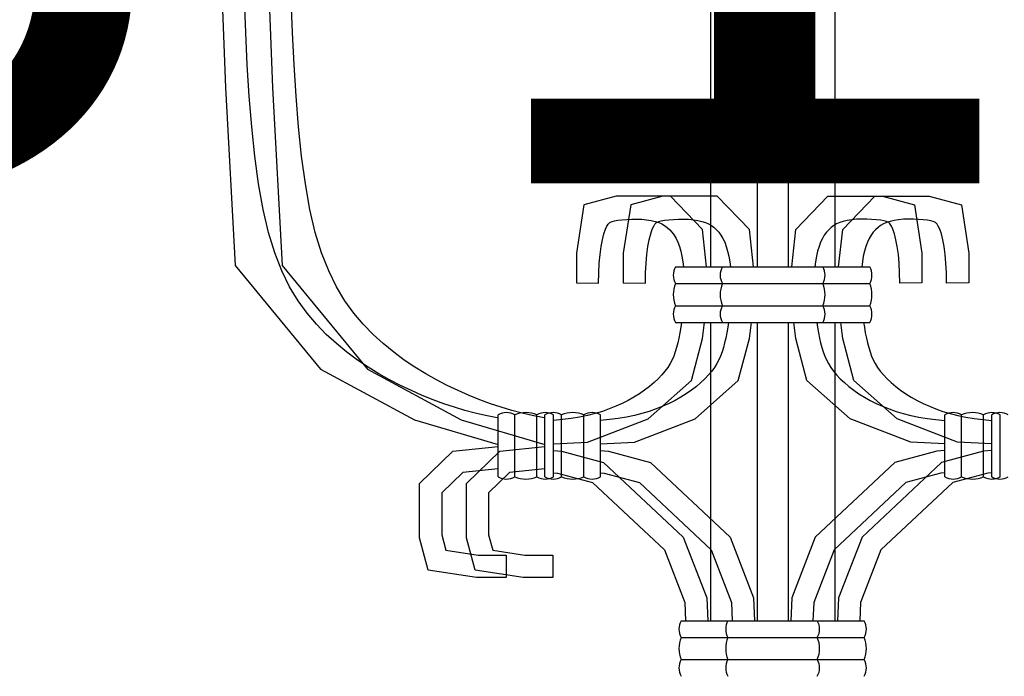
# Model space of a CAD drawing. Units: inches. Extents: x 2278 to 7495, y -71 to 1198.
# Tile 31 of 44: x 5127.04 to 5134.27, y 136.372 to 141.192. Entities that reach past the tile are written whole.
import ezdxf

# ---------------------------------------------------------------- set-up
doc = ezdxf.new("R2010")
doc.units = ezdxf.units.IN
doc.header["$MEASUREMENT"] = 0
doc.layers.add('A-ANNO-DIMS', color=2, linetype='Continuous', lineweight=18)
doc.layers.add('A-ELEV', color=7, linetype='Continuous', lineweight=25)
doc.styles.get("Standard").update_dxf_attribs({"font": 'arial.ttf'})
doc.dimstyles.get("Standard").update_dxf_attribs({"dimtxt": 6, "dimasz": 3, "dimexe": 0.18, "dimexo": 0.0625, "dimgap": 0.09, "dimtad": 0, "dimtih": 1, "dimtoh": 1, "dimdec": 0, "dimzin": 0, "dimdsep": 46, "dimlunit": 3, "dimtxsty": 'Standard', "dimblk": 'ARCHTICK', "dimcen": 0.09, "dimadec": 0, "dimazin": 0, "dimtfac": 1, "dimtdec": 0, "dimtofl": 0, "dimtmove": 0, "dimatfit": 3, "dimfxl": 1, "dimtolj": 1, "dimtzin": 0, "dimarcsym": 0})

# ---------------------------------------------------------------- blocks, each defined once
blk = doc.blocks.new('_ArchTick')
at = {"color": 0, "linetype": 'ByBlock', "const_width": 0.15}
blk.add_lwpolyline([(-0.5, -0.5), (0.5, 0.5)], dxfattribs=at)
blk = doc.blocks.new('*D59')
at = {"layer": 'A-ANNO-DIMS', "color": 0, "lineweight": -2, "transparency": 16777216}
for p, q in [((5096.5894, 159.1826), (5101.5644, 159.1826)), ((5101.3844, 159.1826), (5101.3844, 146.185)), ((5101.3844, 126.7988), (5101.3844, 139.7963)), ((5096.5894, 126.7988), (5101.5644, 126.7988))]:
    blk.add_line(p, q, dxfattribs=at)
at = {"layer": 'Defpoints', "color": 0, "transparency": 16777216}
for p in [(5096.5269, 159.1826), (5101.3844, 159.1826), (5096.5269, 126.7988)]:
    blk.add_point(p, dxfattribs=at)
at = {"layer": 'A-ANNO-DIMS', "color": 0, "lineweight": -2, "transparency": 16777216, "xscale": 3, "yscale": 3, "zscale": 3}
for p, rotation in [((5101.3844, 159.1826), 90), ((5101.3844, 126.7988), 270)]:
    blk.add_blockref('_ArchTick', p, dxfattribs=dict(at, rotation=rotation))
at = {"layer": 'A-ANNO-DIMS', "color": 0, "transparency": 16777216, "insert": (5101.3844, 142.9907), "char_height": 6, "attachment_point": 5}
blk.add_mtext('\\A1;ORNATE BALUSTER 2\'-8 1/2" TYP.', dxfattribs=at)
blk = doc.blocks.new('*D123')
at = {"layer": 'A-ANNO-DIMS', "color": 0, "lineweight": -2, "transparency": 16777216}
for p, q in [((4736.95, 340.1567), (4736.95, -23.4272)), ((5145.6762, -1.8097), (5145.6762, -23.4272)), ((4736.95, -23.2472), (4923.9291, -23.2472)), ((5145.6762, -23.2472), (4958.6971, -23.2472))]:
    blk.add_line(p, q, dxfattribs=at)
at = {"layer": 'Defpoints', "color": 0, "transparency": 16777216}
for p in [(4736.95, 340.2192), (5145.6762, -1.7472), (5145.6762, -23.2472)]:
    blk.add_point(p, dxfattribs=at)
at = {"layer": 'A-ANNO-DIMS', "color": 0, "lineweight": -2, "transparency": 16777216, "xscale": 3, "yscale": 3, "zscale": 3, "rotation": 180}
blk.add_blockref('_ArchTick', (4736.95, -23.2472), dxfattribs=at)
at = {"layer": 'A-ANNO-DIMS', "color": 0, "lineweight": -2, "transparency": 16777216, "xscale": 3, "yscale": 3, "zscale": 3}
blk.add_blockref('_ArchTick', (5145.6762, -23.2472), dxfattribs=at)
at = {"layer": 'A-ANNO-DIMS', "color": 0, "transparency": 16777216, "insert": (4941.3131, -23.2472), "char_height": 6, "attachment_point": 5}
blk.add_mtext('\\A1;34\'-0 1/2"', dxfattribs=at)
blk = doc.blocks.new('*D131')
at = {"layer": 'A-ANNO-DIMS', "color": 0, "lineweight": -2, "transparency": 16777216}
for p, q in [((5096.1762, 99.3153), (5096.1762, 361.8992)), ((5145.6762, 118.3153), (5145.6762, 361.8992)), ((5096.1762, 361.7192), (5105.7503, 361.7192)), ((5145.6762, 361.7192), (5136.1022, 361.7192))]:
    blk.add_line(p, q, dxfattribs=at)
at = {"layer": 'Defpoints', "color": 0, "transparency": 16777216}
for p in [(5145.6762, 361.7192), (5145.6762, 118.2528), (5096.1762, 99.2528)]:
    blk.add_point(p, dxfattribs=at)
at = {"layer": 'A-ANNO-DIMS', "color": 0, "lineweight": -2, "transparency": 16777216, "xscale": 3, "yscale": 3, "zscale": 3, "rotation": 180}
blk.add_blockref('_ArchTick', (5096.1762, 361.7192), dxfattribs=at)
at = {"layer": 'A-ANNO-DIMS', "color": 0, "lineweight": -2, "transparency": 16777216, "xscale": 3, "yscale": 3, "zscale": 3}
blk.add_blockref('_ArchTick', (5145.6762, 361.7192), dxfattribs=at)
at = {"layer": 'A-ANNO-DIMS', "color": 0, "transparency": 16777216, "insert": (5120.9262, 361.7192), "char_height": 6, "attachment_point": 5}
blk.add_mtext('\\A1;4\'-1 1/2"', dxfattribs=at)
blk = doc.blocks.new('*D139')
at = {"layer": 'A-ANNO-DIMS', "color": 0, "lineweight": -2, "transparency": 16777216}
for p, q in [((5092.2387, 160.2528), (5167.7538, 160.2528)), ((5167.5738, 160.2528), (5167.5738, 142.4083)), ((5167.5738, 118.2528), (5167.5738, 136.0973)), ((5145.7387, 118.2528), (5167.7538, 118.2528))]:
    blk.add_line(p, q, dxfattribs=at)
at = {"layer": 'Defpoints', "color": 0, "transparency": 16777216}
for p in [(5092.1762, 160.2528), (5167.5738, 160.2528), (5145.6762, 118.2528)]:
    blk.add_point(p, dxfattribs=at)
at = {"layer": 'A-ANNO-DIMS', "color": 0, "lineweight": -2, "transparency": 16777216, "xscale": 3, "yscale": 3, "zscale": 3}
for p, rotation in [((5167.5738, 160.2528), 90), ((5167.5738, 118.2528), 270)]:
    blk.add_blockref('_ArchTick', p, dxfattribs=dict(at, rotation=rotation))
at = {"layer": 'A-ANNO-DIMS', "color": 0, "transparency": 16777216, "insert": (5167.5738, 139.2528), "char_height": 6, "attachment_point": 5}
blk.add_mtext('\\A1;3\'-6"', dxfattribs=at)

msp = doc.modelspace()

# ---------------------------------------------------------------- linework, layer by layer
at = {"layer": 'A-ELEV'}
for p, q in [((5132.1114, 143.2782), (5132.1114, 139.3773)), ((5132.4553, 143.2782), (5132.4553, 139.3773)), ((5132.6817, 143.2782), (5132.6817, 139.3773)), ((5133.0256, 143.2782), (5133.0256, 139.3773)), ((5128.5267, 141.3278), (5128.5514, 140.694)), ((5128.6994, 141.0971), (5128.6895, 141.3345)), ((5128.8706, 141.3278), (5128.8953, 140.694)), ((5129.0433, 141.0971), (5129.0334, 141.3345)), ((5128.7111, 140.8614), (5128.6994, 141.0971)), ((5129.055, 140.8614), (5129.0433, 141.0971)), ((5128.7255, 140.6297), (5128.7111, 140.8614)), ((5129.0694, 140.6297), (5129.055, 140.8614)), ((5128.5514, 140.694), (5128.6221, 139.3876)), ((5128.7435, 140.4049), (5128.7255, 140.6297)), ((5128.8953, 140.694), (5128.966, 139.3876)), ((5129.0874, 140.4049), (5129.0694, 140.6297)), ((5128.7659, 140.1895), (5128.7435, 140.4049)), ((5129.1098, 140.1895), (5129.0874, 140.4049)), ((5128.7934, 139.9866), (5128.7659, 140.1895)), ((5129.1373, 139.9866), (5129.1098, 140.1895)), ((5128.8267, 139.799), (5128.7934, 139.9866)), ((5129.1706, 139.799), (5129.1373, 139.9866)), ((5131.1826, 139.8322), (5131.1281, 139.4783)), ((5131.4186, 139.8957), (5131.1826, 139.8322)), ((5131.8181, 139.8957), (5131.4186, 139.8957)), ((5131.5265, 139.8322), (5131.472, 139.4783)), ((5131.7625, 139.8957), (5131.5265, 139.8322)), ((5132.162, 139.8957), (5131.7625, 139.8957)), ((5132.0542, 139.6507), (5131.8181, 139.8957)), ((5132.3981, 139.6507), (5132.162, 139.8957)), ((5132.7389, 139.6507), (5132.975, 139.8957)), ((5132.975, 139.8957), (5133.3745, 139.8957)), ((5133.0828, 139.6507), (5133.3189, 139.8957)), ((5133.3189, 139.8957), (5133.7184, 139.8957)), ((5133.3745, 139.8957), (5133.6106, 139.8322)), ((5133.6106, 139.8322), (5133.6651, 139.4783)), ((5133.7184, 139.8957), (5133.9545, 139.8322)), ((5133.9545, 139.8322), (5134.009, 139.4783)), ((5128.8662, 139.6298), (5128.8267, 139.799)), ((5129.2101, 139.6298), (5129.1706, 139.799)), ((5131.352, 139.6768), (5131.3607, 139.6907)), ((5131.3607, 139.6907), (5131.367, 139.698)), ((5131.367, 139.698), (5131.3721, 139.7021)), ((5131.3721, 139.7021), (5131.3786, 139.7059)), ((5131.3786, 139.7059), (5131.3895, 139.7102)), ((5131.3895, 139.7102), (5131.4069, 139.7149)), ((5131.4069, 139.7149), (5131.4313, 139.7192)), ((5131.4313, 139.7192), (5131.4623, 139.7229)), ((5131.4623, 139.7229), (5131.4975, 139.7259)), ((5131.4975, 139.7259), (5131.5342, 139.7277)), ((5131.5342, 139.7277), (5131.5713, 139.728)), ((5131.5713, 139.728), (5131.6079, 139.7266)), ((5131.6079, 139.7266), (5131.6431, 139.7233)), ((5131.6431, 139.7233), (5131.6761, 139.7182)), ((5131.6761, 139.7182), (5131.7059, 139.7113)), ((5131.6959, 139.6768), (5131.7046, 139.6907)), ((5131.7046, 139.6907), (5131.7109, 139.698)), ((5131.7059, 139.7113), (5131.732, 139.7027)), ((5131.7109, 139.698), (5131.716, 139.7021)), ((5131.716, 139.7021), (5131.7225, 139.7059)), ((5131.7225, 139.7059), (5131.7334, 139.7102)), ((5131.732, 139.7027), (5131.7548, 139.6925)), ((5131.7334, 139.7102), (5131.7508, 139.7149)), ((5131.7508, 139.7149), (5131.7753, 139.7192)), ((5131.7548, 139.6925), (5131.7756, 139.6804)), ((5131.7753, 139.7192), (5131.8062, 139.7229)), ((5131.8062, 139.7229), (5131.8414, 139.7259)), ((5131.8414, 139.7259), (5131.8781, 139.7277)), ((5131.8781, 139.7277), (5131.9152, 139.728)), ((5131.9152, 139.728), (5131.9518, 139.7266)), ((5131.9518, 139.7266), (5131.987, 139.7233)), ((5131.987, 139.7233), (5132.02, 139.7182)), ((5132.02, 139.7182), (5132.0498, 139.7113)), ((5132.0498, 139.7113), (5132.0759, 139.7027)), ((5132.0759, 139.7027), (5132.0987, 139.6925)), ((5132.0987, 139.6925), (5132.1195, 139.6804)), ((5133.0383, 139.6925), (5133.0176, 139.6804)), ((5133.0611, 139.7027), (5133.0383, 139.6925)), ((5133.0872, 139.7113), (5133.0611, 139.7027)), ((5133.117, 139.7182), (5133.0872, 139.7113)), ((5133.15, 139.7233), (5133.117, 139.7182)), ((5133.1853, 139.7266), (5133.15, 139.7233)), ((5133.2219, 139.728), (5133.1853, 139.7266)), ((5133.259, 139.7277), (5133.2219, 139.728)), ((5133.2957, 139.7259), (5133.259, 139.7277)), ((5133.3308, 139.7229), (5133.2957, 139.7259)), ((5133.3618, 139.7192), (5133.3308, 139.7229)), ((5133.3822, 139.6925), (5133.3615, 139.6804)), ((5133.3862, 139.7149), (5133.3618, 139.7192)), ((5133.405, 139.7027), (5133.3822, 139.6925)), ((5133.4036, 139.7102), (5133.3862, 139.7149)), ((5133.4146, 139.7059), (5133.4036, 139.7102)), ((5133.4311, 139.7113), (5133.405, 139.7027)), ((5133.4211, 139.7021), (5133.4146, 139.7059)), ((5133.4261, 139.698), (5133.4211, 139.7021)), ((5133.4324, 139.6907), (5133.4261, 139.698)), ((5133.4609, 139.7182), (5133.4311, 139.7113)), ((5133.4411, 139.6768), (5133.4324, 139.6907)), ((5133.4939, 139.7233), (5133.4609, 139.7182)), ((5133.5292, 139.7266), (5133.4939, 139.7233)), ((5133.5658, 139.728), (5133.5292, 139.7266)), ((5133.6029, 139.7277), (5133.5658, 139.728)), ((5133.6396, 139.7259), (5133.6029, 139.7277)), ((5133.6747, 139.7229), (5133.6396, 139.7259)), ((5133.7057, 139.7192), (5133.6747, 139.7229)), ((5133.7301, 139.7149), (5133.7057, 139.7192)), ((5133.7475, 139.7102), (5133.7301, 139.7149)), ((5133.7585, 139.7059), (5133.7475, 139.7102)), ((5133.765, 139.7021), (5133.7585, 139.7059)), ((5133.77, 139.698), (5133.765, 139.7021)), ((5133.7763, 139.6907), (5133.77, 139.698)), ((5133.785, 139.6768), (5133.7763, 139.6907)), ((5128.9124, 139.4803), (5128.8662, 139.6298)), ((5129.2563, 139.4803), (5129.2101, 139.6298)), ((5131.3188, 139.5767), (5131.3297, 139.6195)), ((5131.3297, 139.6195), (5131.3412, 139.6532)), ((5131.3412, 139.6532), (5131.352, 139.6768)), ((5131.6627, 139.5767), (5131.6736, 139.6195)), ((5131.6736, 139.6195), (5131.6851, 139.6532)), ((5131.6851, 139.6532), (5131.6959, 139.6768)), ((5131.7756, 139.6804), (5131.7948, 139.6662)), ((5131.7948, 139.6662), (5131.8127, 139.6499)), ((5131.8127, 139.6499), (5131.8294, 139.6311)), ((5131.8294, 139.6311), (5131.845, 139.6096)), ((5132.0839, 139.3773), (5132.0542, 139.6507)), ((5132.1195, 139.6804), (5132.1387, 139.6662)), ((5132.1387, 139.6662), (5132.1566, 139.6499)), ((5132.1566, 139.6499), (5132.1733, 139.6311)), ((5132.1733, 139.6311), (5132.1889, 139.6096)), ((5132.4278, 139.3773), (5132.3981, 139.6507)), ((5132.7092, 139.3773), (5132.7389, 139.6507)), ((5132.9637, 139.6311), (5132.9481, 139.6096)), ((5132.9805, 139.6499), (5132.9637, 139.6311)), ((5132.9984, 139.6662), (5132.9805, 139.6499)), ((5133.0176, 139.6804), (5132.9984, 139.6662)), ((5133.0531, 139.3773), (5133.0828, 139.6507)), ((5133.3076, 139.6311), (5133.292, 139.6096)), ((5133.3244, 139.6499), (5133.3076, 139.6311)), ((5133.3423, 139.6662), (5133.3244, 139.6499)), ((5133.3615, 139.6804), (5133.3423, 139.6662)), ((5133.4519, 139.6532), (5133.4411, 139.6768)), ((5133.4634, 139.6195), (5133.4519, 139.6532)), ((5133.4743, 139.5767), (5133.4634, 139.6195)), ((5133.7958, 139.6532), (5133.785, 139.6768)), ((5133.8073, 139.6195), (5133.7958, 139.6532)), ((5133.8182, 139.5767), (5133.8073, 139.6195)), ((5131.3092, 139.526), (5131.3188, 139.5767)), ((5131.6531, 139.526), (5131.6627, 139.5767)), ((5131.845, 139.6096), (5131.8594, 139.5853)), ((5131.8594, 139.5853), (5131.8724, 139.558)), ((5131.8724, 139.558), (5131.884, 139.5272)), ((5132.1889, 139.6096), (5132.2033, 139.5853)), ((5132.2033, 139.5853), (5132.2163, 139.558)), ((5132.2163, 139.558), (5132.2279, 139.5272)), ((5132.9207, 139.558), (5132.9091, 139.5272)), ((5132.9337, 139.5853), (5132.9207, 139.558)), ((5132.9481, 139.6096), (5132.9337, 139.5853)), ((5133.2646, 139.558), (5133.253, 139.5272)), ((5133.2776, 139.5853), (5133.2646, 139.558)), ((5133.292, 139.6096), (5133.2776, 139.5853)), ((5133.4839, 139.526), (5133.4743, 139.5767)), ((5133.8278, 139.526), (5133.8182, 139.5767)), ((5128.9646, 139.3484), (5128.9124, 139.4803)), ((5129.3085, 139.3484), (5129.2563, 139.4803)), ((5131.1281, 139.4783), (5131.1281, 139.2606)), ((5131.3015, 139.4682), (5131.3092, 139.526)), ((5131.472, 139.4783), (5131.472, 139.2606)), ((5131.6454, 139.4682), (5131.6531, 139.526)), ((5131.884, 139.5272), (5131.8942, 139.4929)), ((5131.8942, 139.4929), (5131.9029, 139.4553)), ((5132.2279, 139.5272), (5132.2381, 139.4929)), ((5132.2381, 139.4929), (5132.2468, 139.4553)), ((5132.8989, 139.4929), (5132.8903, 139.4553)), ((5132.9091, 139.5272), (5132.8989, 139.4929)), ((5133.2428, 139.4929), (5133.2342, 139.4553)), ((5133.253, 139.5272), (5133.2428, 139.4929)), ((5133.4917, 139.4682), (5133.4839, 139.526)), ((5133.6651, 139.4783), (5133.6651, 139.2606)), ((5133.8356, 139.4682), (5133.8278, 139.526)), ((5134.009, 139.4783), (5134.009, 139.2606)), ((5131.2922, 139.3348), (5131.2957, 139.4043)), ((5131.2957, 139.4043), (5131.3015, 139.4682)), ((5131.6361, 139.3348), (5131.6396, 139.4043)), ((5131.6396, 139.4043), (5131.6454, 139.4682)), ((5131.9029, 139.4553), (5131.9098, 139.4152)), ((5131.9098, 139.4152), (5131.9146, 139.3773)), ((5132.2468, 139.4553), (5132.2537, 139.4152)), ((5132.2537, 139.4152), (5132.2585, 139.3773)), ((5132.8833, 139.4152), (5132.8786, 139.3773)), ((5132.8903, 139.4553), (5132.8833, 139.4152)), ((5133.2272, 139.4152), (5133.2225, 139.3773)), ((5133.2342, 139.4553), (5133.2272, 139.4152)), ((5133.4974, 139.4043), (5133.4917, 139.4682)), ((5133.5009, 139.3348), (5133.4974, 139.4043)), ((5133.8413, 139.4043), (5133.8356, 139.4682)), ((5133.8448, 139.3348), (5133.8413, 139.4043)), ((5128.6221, 139.3876), (5129.2486, 138.6255)), ((5129.0219, 139.2321), (5128.9646, 139.3484)), ((5128.966, 139.3876), (5129.5925, 138.6255)), ((5129.3658, 139.2321), (5129.3085, 139.3484)), ((5131.291, 139.258), (5131.2922, 139.3348)), ((5131.6349, 139.258), (5131.6361, 139.3348)), ((5131.8558, 139.3773), (5132.9373, 139.3773)), ((5132.1997, 139.3773), (5133.2812, 139.3773)), ((5133.5021, 139.258), (5133.5009, 139.3348)), ((5133.846, 139.258), (5133.8448, 139.3348)), ((5131.1281, 139.2606), (5131.291, 139.258)), ((5131.472, 139.2606), (5131.6349, 139.258)), ((5131.8558, 139.2551), (5132.9373, 139.2551)), ((5132.1997, 139.2551), (5133.2812, 139.2551)), ((5133.6651, 139.2606), (5133.5021, 139.258)), ((5134.009, 139.2606), (5133.846, 139.258)), ((5129.0837, 139.1293), (5129.0219, 139.2321)), ((5129.4276, 139.1293), (5129.3658, 139.2321)), ((5129.1494, 139.038), (5129.0837, 139.1293)), ((5129.4933, 139.038), (5129.4276, 139.1293)), ((5129.2186, 138.9562), (5129.1494, 139.038)), ((5129.5625, 138.9562), (5129.4933, 139.038)), ((5131.8558, 139.0921), (5132.9373, 139.0921)), ((5132.1997, 139.0921), (5133.2812, 139.0921)), ((5131.8558, 138.9699), (5132.9373, 138.9699)), ((5131.9005, 138.9699), (5131.895, 138.9347)), ((5132.0542, 138.8523), (5132.0682, 138.9699)), ((5132.1114, 138.9699), (5132.1114, 136.779)), ((5132.1997, 138.9699), (5133.2812, 138.9699)), ((5132.2444, 138.9699), (5132.2389, 138.9347)), ((5132.3981, 138.8523), (5132.4121, 138.9699)), ((5132.4553, 138.9699), (5132.4553, 136.779)), ((5132.6817, 138.9699), (5132.6817, 136.779)), ((5132.7389, 138.8523), (5132.7249, 138.9699)), ((5132.8926, 138.9699), (5132.8981, 138.9347)), ((5133.0256, 138.9699), (5133.0256, 136.779)), ((5133.0828, 138.8523), (5133.0688, 138.9699)), ((5133.2365, 138.9699), (5133.242, 138.9347)), ((5129.2908, 138.882), (5129.2186, 138.9562)), ((5129.6347, 138.882), (5129.5625, 138.9562)), ((5131.8879, 138.8941), (5131.8803, 138.8552)), ((5131.895, 138.9347), (5131.8879, 138.8941)), ((5132.2318, 138.8941), (5132.2242, 138.8552)), ((5132.2389, 138.9347), (5132.2318, 138.8941)), ((5132.8981, 138.9347), (5132.9052, 138.8941)), ((5132.9052, 138.8941), (5132.9128, 138.8552)), ((5133.242, 138.9347), (5133.2491, 138.8941)), ((5133.2491, 138.8941), (5133.2567, 138.8552)), ((5129.3657, 138.8139), (5129.2908, 138.882)), ((5129.7096, 138.8139), (5129.6347, 138.882)), ((5131.8722, 138.8187), (5131.8633, 138.7847)), ((5131.8803, 138.8552), (5131.8722, 138.8187)), ((5131.9725, 138.5439), (5132.0542, 138.8523)), ((5132.2161, 138.8187), (5132.2072, 138.7847)), ((5132.2242, 138.8552), (5132.2161, 138.8187)), ((5132.3164, 138.5439), (5132.3981, 138.8523)), ((5132.8207, 138.5439), (5132.7389, 138.8523)), ((5132.9128, 138.8552), (5132.9209, 138.8187)), ((5132.9209, 138.8187), (5132.9298, 138.7847)), ((5133.1646, 138.5439), (5133.0828, 138.8523)), ((5133.2567, 138.8552), (5133.2648, 138.8187)), ((5133.2648, 138.8187), (5133.2737, 138.7847)), ((5129.4423, 138.751), (5129.3657, 138.8139)), ((5129.5199, 138.6933), (5129.4423, 138.751)), ((5129.7862, 138.751), (5129.7096, 138.8139)), ((5129.8638, 138.6933), (5129.7862, 138.751)), ((5131.8534, 138.7528), (5131.8422, 138.7228)), ((5131.8633, 138.7847), (5131.8534, 138.7528)), ((5132.1973, 138.7528), (5132.1861, 138.7228)), ((5132.2072, 138.7847), (5132.1973, 138.7528)), ((5132.9298, 138.7847), (5132.9397, 138.7528)), ((5132.9397, 138.7528), (5132.9509, 138.7228)), ((5133.2737, 138.7847), (5133.2836, 138.7528)), ((5133.2836, 138.7528), (5133.2948, 138.7228)), ((5129.598, 138.6404), (5129.5199, 138.6933)), ((5129.942, 138.6404), (5129.8638, 138.6933)), ((5131.8296, 138.6944), (5131.815, 138.6669)), ((5131.8422, 138.7228), (5131.8296, 138.6944)), ((5132.1735, 138.6944), (5132.159, 138.6669)), ((5132.1861, 138.7228), (5132.1735, 138.6944)), ((5132.9509, 138.7228), (5132.9635, 138.6944)), ((5132.9635, 138.6944), (5132.9781, 138.6669)), ((5133.2948, 138.7228), (5133.3074, 138.6944)), ((5133.3074, 138.6944), (5133.322, 138.6669)), ((5129.2486, 138.6255), (5129.9387, 138.2535)), ((5129.5925, 138.6255), (5130.2826, 138.2535)), ((5129.6768, 138.5919), (5129.598, 138.6404)), ((5130.0207, 138.5919), (5129.942, 138.6404)), ((5131.7781, 138.6124), (5131.7545, 138.5843)), ((5131.7981, 138.6398), (5131.7781, 138.6124)), ((5131.815, 138.6669), (5131.7981, 138.6398)), ((5132.122, 138.6124), (5132.0984, 138.5843)), ((5132.142, 138.6398), (5132.122, 138.6124)), ((5132.159, 138.6669), (5132.142, 138.6398)), ((5132.9781, 138.6669), (5132.995, 138.6398)), ((5132.995, 138.6398), (5133.0151, 138.6124)), ((5133.0151, 138.6124), (5133.0386, 138.5843)), ((5133.322, 138.6669), (5133.3389, 138.6398)), ((5133.3389, 138.6398), (5133.359, 138.6124)), ((5133.359, 138.6124), (5133.3825, 138.5843)), ((5129.7561, 138.5474), (5129.6768, 138.5919)), ((5129.8357, 138.5065), (5129.7561, 138.5474)), ((5130.1, 138.5474), (5130.0207, 138.5919)), ((5130.1796, 138.5065), (5130.1, 138.5474)), ((5131.6547, 138.2626), (5131.9725, 138.5439)), ((5131.7276, 138.556), (5131.6975, 138.5277)), ((5131.7545, 138.5843), (5131.7276, 138.556)), ((5131.9986, 138.2626), (5132.3164, 138.5439)), ((5132.0715, 138.556), (5132.0414, 138.5277)), ((5132.0984, 138.5843), (5132.0715, 138.556)), ((5133.1384, 138.2626), (5132.8207, 138.5439)), ((5133.0386, 138.5843), (5133.0655, 138.556)), ((5133.0655, 138.556), (5133.0956, 138.5277)), ((5133.4823, 138.2626), (5133.1646, 138.5439)), ((5133.3825, 138.5843), (5133.4094, 138.556)), ((5133.4094, 138.556), (5133.4395, 138.5277)), ((5129.9156, 138.4689), (5129.8357, 138.5065)), ((5129.9956, 138.4341), (5129.9156, 138.4689)), ((5130.2595, 138.4689), (5130.1796, 138.5065)), ((5130.3395, 138.4341), (5130.2595, 138.4689)), ((5131.6288, 138.4725), (5131.5906, 138.4461)), ((5131.6645, 138.4998), (5131.6288, 138.4725)), ((5131.6975, 138.5277), (5131.6645, 138.4998)), ((5131.9727, 138.4725), (5131.9345, 138.4461)), ((5132.0084, 138.4998), (5131.9727, 138.4725)), ((5132.0414, 138.5277), (5132.0084, 138.4998)), ((5133.0956, 138.5277), (5133.1286, 138.4998)), ((5133.1286, 138.4998), (5133.1644, 138.4725)), ((5133.1644, 138.4725), (5133.2026, 138.4461)), ((5133.4395, 138.5277), (5133.4725, 138.4998)), ((5133.4725, 138.4998), (5133.5083, 138.4725)), ((5133.5083, 138.4725), (5133.5465, 138.4461)), ((5130.0751, 138.402), (5129.9956, 138.4341)), ((5130.1538, 138.3729), (5130.0751, 138.402)), ((5130.419, 138.402), (5130.3395, 138.4341)), ((5130.4977, 138.3729), (5130.419, 138.402)), ((5131.5079, 138.397), (5131.4637, 138.3746)), ((5131.5502, 138.4208), (5131.5079, 138.397)), ((5131.5906, 138.4461), (5131.5502, 138.4208)), ((5131.8518, 138.397), (5131.8076, 138.3746)), ((5131.8941, 138.4208), (5131.8518, 138.397)), ((5131.9345, 138.4461), (5131.8941, 138.4208)), ((5133.2026, 138.4461), (5133.2429, 138.4208)), ((5133.2429, 138.4208), (5133.2852, 138.397)), ((5133.2852, 138.397), (5133.3294, 138.3746)), ((5133.5465, 138.4461), (5133.5868, 138.4208)), ((5133.5868, 138.4208), (5133.6291, 138.397)), ((5133.6291, 138.397), (5133.6733, 138.3746)), ((5130.2316, 138.3466), (5130.1538, 138.3729)), ((5130.3086, 138.3234), (5130.2316, 138.3466)), ((5130.3846, 138.3031), (5130.3086, 138.3234)), ((5130.5755, 138.3466), (5130.4977, 138.3729)), ((5130.6525, 138.3234), (5130.5755, 138.3466)), ((5130.7285, 138.3031), (5130.6525, 138.3234)), ((5131.3184, 138.3168), (5131.2652, 138.3009)), ((5131.3691, 138.3345), (5131.3184, 138.3168)), ((5131.4175, 138.3537), (5131.3691, 138.3345)), ((5131.4637, 138.3746), (5131.4175, 138.3537)), ((5131.6623, 138.3168), (5131.6091, 138.3009)), ((5131.713, 138.3345), (5131.6623, 138.3168)), ((5131.7614, 138.3537), (5131.713, 138.3345)), ((5131.8076, 138.3746), (5131.7614, 138.3537)), ((5133.3294, 138.3746), (5133.3756, 138.3537)), ((5133.3756, 138.3537), (5133.424, 138.3345)), ((5133.424, 138.3345), (5133.4747, 138.3168)), ((5133.4747, 138.3168), (5133.5279, 138.3009)), ((5133.6733, 138.3746), (5133.7195, 138.3537)), ((5133.7195, 138.3537), (5133.7679, 138.3345)), ((5133.7679, 138.3345), (5133.8186, 138.3168)), ((5133.8186, 138.3168), (5133.8718, 138.3009)), ((5129.9387, 138.2535), (5130.5528, 138.0746)), ((5130.2826, 138.2535), (5130.8967, 138.0746)), ((5130.4597, 138.286), (5130.3846, 138.3031)), ((5130.5338, 138.2719), (5130.4597, 138.286)), ((5130.5528, 138.2691), (5130.5338, 138.2719)), ((5130.5528, 137.8357), (5130.5528, 138.2916)), ((5130.675, 137.8357), (5130.675, 138.2916)), ((5130.8036, 138.286), (5130.7285, 138.3031)), ((5130.8777, 138.2719), (5130.8036, 138.286)), ((5130.838, 137.8357), (5130.838, 138.2916)), ((5130.8967, 138.2691), (5130.8777, 138.2719)), ((5130.8967, 137.8357), (5130.8967, 138.2916)), ((5130.9602, 137.8357), (5130.9602, 138.2916)), ((5131.0258, 138.2562), (5130.9602, 138.2505)), ((5131.0189, 137.8357), (5131.0189, 138.2916)), ((5131.0896, 138.2644), (5131.0258, 138.2562)), ((5131.1509, 138.2746), (5131.0896, 138.2644)), ((5131.2094, 138.2868), (5131.1509, 138.2746)), ((5131.1819, 137.8357), (5131.1819, 138.2916)), ((5131.2652, 138.3009), (5131.2094, 138.2868)), ((5131.2098, 138.0902), (5131.6547, 138.2626)), ((5131.3041, 137.8357), (5131.3041, 138.2916)), ((5131.3697, 138.2562), (5131.3041, 138.2505)), ((5131.4335, 138.2644), (5131.3697, 138.2562)), ((5131.4948, 138.2746), (5131.4335, 138.2644)), ((5131.5534, 138.2868), (5131.4948, 138.2746)), ((5131.6091, 138.3009), (5131.5534, 138.2868)), ((5131.5537, 138.0902), (5131.9986, 138.2626)), ((5133.5833, 138.0902), (5133.1384, 138.2626)), ((5133.9272, 138.0902), (5133.4823, 138.2626)), ((5133.5279, 138.3009), (5133.5837, 138.2868)), ((5133.5837, 138.2868), (5133.6422, 138.2746)), ((5133.6422, 138.2746), (5133.7035, 138.2644)), ((5133.7035, 138.2644), (5133.7673, 138.2562)), ((5133.7673, 138.2562), (5133.833, 138.2505)), ((5133.833, 137.8357), (5133.833, 138.2916)), ((5133.8718, 138.3009), (5133.9276, 138.2868)), ((5133.9276, 138.2868), (5133.9861, 138.2746)), ((5133.9552, 137.8357), (5133.9552, 138.2916)), ((5133.9861, 138.2746), (5134.0474, 138.2644)), ((5134.0474, 138.2644), (5134.1112, 138.2562)), ((5134.1112, 138.2562), (5134.1769, 138.2505)), ((5134.1181, 137.8357), (5134.1181, 138.2916)), ((5134.1769, 137.8357), (5134.1769, 138.2916)), ((5134.2403, 137.8357), (5134.2403, 138.2916)), ((5129.9756, 137.7875), (5130.2206, 138.0235)), ((5130.2206, 138.0235), (5130.5528, 138.0597)), ((5130.3195, 137.7875), (5130.5645, 138.0235)), ((5130.5645, 138.0235), (5130.8967, 138.0597)), ((5130.9602, 138.0792), (5131.2098, 138.0902)), ((5130.9602, 138.0306), (5131.019, 138.0235)), ((5131.019, 138.0235), (5131.3274, 137.9418)), ((5131.3041, 138.0792), (5131.5537, 138.0902)), ((5131.3041, 138.0306), (5131.3629, 138.0235)), ((5131.3629, 138.0235), (5131.6713, 137.9418)), ((5133.7742, 138.0235), (5133.4657, 137.9418)), ((5133.833, 138.0792), (5133.5833, 138.0902)), ((5133.833, 138.0306), (5133.7742, 138.0235)), ((5134.1181, 138.0235), (5133.8096, 137.9418)), ((5134.1769, 138.0792), (5133.9272, 138.0902)), ((5134.1769, 138.0306), (5134.1181, 138.0235)), ((5130.5528, 137.8958), (5130.2936, 137.8676)), ((5130.8967, 137.8958), (5130.6375, 137.8676)), ((5131.3274, 137.9418), (5131.9118, 137.3933)), ((5131.6713, 137.9418), (5132.2557, 137.3933)), ((5133.4657, 137.9418), (5132.8813, 137.3933)), ((5133.8096, 137.9418), (5133.2252, 137.3933)), ((5130.2936, 137.8676), (5130.1386, 137.7182)), ((5130.6375, 137.8676), (5130.4825, 137.7182)), ((5130.9602, 137.8665), (5130.9883, 137.8631)), ((5130.9883, 137.8631), (5131.2459, 137.7949)), ((5131.3041, 137.8665), (5131.3322, 137.8631)), ((5131.3322, 137.8631), (5131.5898, 137.7949)), ((5133.8048, 137.8631), (5133.5472, 137.7949)), ((5133.833, 137.8665), (5133.8048, 137.8631)), ((5134.1487, 137.8631), (5133.8911, 137.7949)), ((5134.1769, 137.8665), (5134.1487, 137.8631)), ((5129.9756, 137.388), (5129.9756, 137.7875)), ((5130.3195, 137.388), (5130.3195, 137.7875)), ((5131.2459, 137.7949), (5131.7733, 137.2998)), ((5131.5898, 137.7949), (5132.1172, 137.2998)), ((5133.5472, 137.7949), (5133.0199, 137.2998)), ((5133.8911, 137.7949), (5133.3638, 137.2998)), ((5130.1386, 137.7182), (5130.1386, 137.4095)), ((5130.4825, 137.7182), (5130.4825, 137.4095)), ((5130.0391, 137.1519), (5129.9756, 137.388)), ((5130.1386, 137.4095), (5130.1689, 137.2968)), ((5130.383, 137.1519), (5130.3195, 137.388)), ((5130.4825, 137.4095), (5130.5128, 137.2968)), ((5131.9118, 137.3933), (5132.0842, 136.9484)), ((5132.2557, 137.3933), (5132.4281, 136.9484)), ((5132.8813, 137.3933), (5132.7089, 136.9484)), ((5133.2252, 137.3933), (5133.0528, 136.9484)), ((5131.7733, 137.2998), (5131.9226, 136.9144)), ((5132.1172, 137.2998), (5132.2665, 136.9144)), ((5133.0199, 137.2998), (5132.8705, 136.9144)), ((5133.3638, 137.2998), (5133.2144, 136.9144)), ((5130.1689, 137.2968), (5130.4054, 137.2604)), ((5130.4054, 137.2604), (5130.6107, 137.2604)), ((5130.5128, 137.2968), (5130.7493, 137.2604)), ((5130.6107, 137.2604), (5130.6107, 137.0974)), ((5130.7493, 137.2604), (5130.9546, 137.2604)), ((5130.9546, 137.2604), (5130.9546, 137.0974)), ((5130.393, 137.0974), (5130.0391, 137.1519)), ((5130.7369, 137.0974), (5130.383, 137.1519)), ((5130.6107, 137.0974), (5130.393, 137.0974)), ((5130.9546, 137.0974), (5130.7369, 137.0974)), ((5132.0842, 136.9484), (5132.0917, 136.779)), ((5132.4281, 136.9484), (5132.4356, 136.779)), ((5132.7089, 136.9484), (5132.7015, 136.779)), ((5133.0528, 136.9484), (5133.0454, 136.779)), ((5131.9226, 136.9144), (5131.9286, 136.779)), ((5132.2665, 136.9144), (5132.2725, 136.779)), ((5132.8705, 136.9144), (5132.8646, 136.779)), ((5133.2144, 136.9144), (5133.2085, 136.779)), ((5131.8965, 136.779), (5132.8966, 136.779)), ((5132.2404, 136.779), (5133.2405, 136.779)), ((5131.8965, 136.6568), (5132.8966, 136.6568)), ((5132.2404, 136.6568), (5133.2405, 136.6568)), ((5131.8965, 136.4939), (5132.8966, 136.4939)), ((5132.2404, 136.4939), (5133.2405, 136.4939))]:
    msp.add_line(p, q, dxfattribs=at)
for centre, radius, start, end in [((5131.9607, 139.3162), 0.1214, 149.77678, 210.22322), ((5132.3046, 139.3162), 0.1214, 149.77678, 210.22322), ((5132.8324, 139.3162), 0.1214, 329.77678, 30.22322), ((5133.1764, 139.3162), 0.1214, 329.77678, 30.22322), ((5132.0487, 139.1736), 0.2094, 157.10166, 202.89834), ((5132.3926, 139.1736), 0.2094, 157.10166, 202.89834), ((5132.7445, 139.1736), 0.2094, 337.10166, 22.89834), ((5133.0884, 139.1736), 0.2094, 337.10166, 22.89834), ((5131.9607, 139.031), 0.1214, 149.77678, 210.22322), ((5132.3046, 139.031), 0.1214, 149.77678, 210.22322), ((5132.8324, 139.031), 0.1214, 329.77678, 30.22322), ((5133.1764, 139.031), 0.1214, 329.77678, 30.22322), ((5130.6139, 138.1867), 0.1214, 59.77678, 120.22322), ((5130.7565, 138.0987), 0.2094, 67.10166, 112.89834), ((5130.8991, 138.1867), 0.1214, 59.77678, 120.22322), ((5130.9578, 138.1867), 0.1214, 59.77678, 120.22322), ((5131.1004, 138.0987), 0.2094, 67.10166, 112.89834), ((5131.243, 138.1867), 0.1214, 59.77678, 120.22322), ((5133.8941, 138.1867), 0.1214, 59.77678, 120.22322), ((5134.0366, 138.0987), 0.2094, 67.10166, 112.89834), ((5134.1792, 138.1867), 0.1214, 59.77678, 120.22322), ((5134.238, 138.1867), 0.1214, 59.77678, 120.22322), ((5130.6139, 137.9406), 0.1214, 239.77678, 300.22322), ((5130.7565, 138.0286), 0.2094, 247.10166, 292.89834), ((5130.8991, 137.9406), 0.1214, 239.77678, 300.22322), ((5130.9578, 137.9406), 0.1214, 239.77678, 300.22322), ((5131.1004, 138.0286), 0.2094, 247.10166, 292.89834), ((5131.243, 137.9406), 0.1214, 239.77678, 300.22322), ((5133.8941, 137.9406), 0.1214, 239.77678, 300.22322), ((5134.0366, 138.0286), 0.2094, 247.10166, 292.89834), ((5134.1792, 137.9406), 0.1214, 239.77678, 300.22322), ((5134.238, 137.9406), 0.1214, 239.77678, 300.22322), ((5132.0014, 136.7179), 0.1214, 149.77678, 210.22322), ((5132.3453, 136.7179), 0.1214, 149.77678, 210.22322), ((5132.7917, 136.7179), 0.1214, 329.77678, 30.22322), ((5133.1356, 136.7179), 0.1214, 329.77678, 30.22322), ((5132.0894, 136.5754), 0.2094, 157.10166, 202.89834), ((5132.4333, 136.5754), 0.2094, 157.10166, 202.89834), ((5132.7037, 136.5754), 0.2094, 337.10166, 22.89834), ((5133.0476, 136.5754), 0.2094, 337.10166, 22.89834), ((5132.0014, 136.4328), 0.1214, 149.77678, 210.22322), ((5132.3453, 136.4328), 0.1214, 149.77678, 210.22322), ((5132.7917, 136.4328), 0.1214, 329.77678, 30.22322), ((5133.1356, 136.4328), 0.1214, 329.77678, 30.22322)]:
    msp.add_arc(centre, radius, start, end, dxfattribs=at)

# ---------------------------------------------------------------- dimensions: what is measured, and where the dimension line sits
at = {"layer": 'A-ANNO-DIMS'}
for base, p1, p2, picture, middle in [((5145.6762, 361.7192), (5096.1762, 99.2528), (5145.6762, 118.2528), '*D131', (5120.9262, 361.7192)), ((5145.6762, -23.2472), (4736.95, 340.2192), (5145.6762, -1.7472), '*D123', (4941.3131, -23.2472))]:
    dim = msp.add_linear_dim(base=base, p1=p1, p2=p2, dimstyle='Standard', override={"dimdec": 1, "dimlfac": 1, "dimrnd": 0, "dimzin": 1, "dimdsep": 46, "dimlunit": 4, "dimfrac": 2}, dxfattribs=at)
    dim.commit()
    dim.dimension.update_dxf_attribs({"geometry": picture, "text_midpoint": middle})
dim = msp.add_linear_dim(base=(5101.3844, 159.1826), p1=(5096.5269, 126.7988), p2=(5096.5269, 159.1826), angle=90, text='ORNATE BALUSTER <> TYP.', dimstyle='Standard', override={"dimdec": 1, "dimrnd": 0, "dimzin": 1, "dimlunit": 4, "dimfrac": 2}, dxfattribs=at)
dim.commit()
dim.dimension.update_dxf_attribs({"geometry": '*D59', "text_midpoint": (5101.3844, 142.9907)})
dim = msp.add_linear_dim(base=(5167.5738, 160.2528), p1=(5145.6762, 118.2528), p2=(5092.1762, 160.2528), angle=90, dimstyle='Standard', override={"dimdec": 1, "dimlfac": 1, "dimrnd": 0, "dimzin": 1, "dimdsep": 46, "dimlunit": 4, "dimfrac": 2}, dxfattribs=at)
dim.commit()
dim.dimension.update_dxf_attribs({"geometry": '*D139', "text_midpoint": (5167.5738, 139.2528)})

doc.saveas('drawing.dxf')
